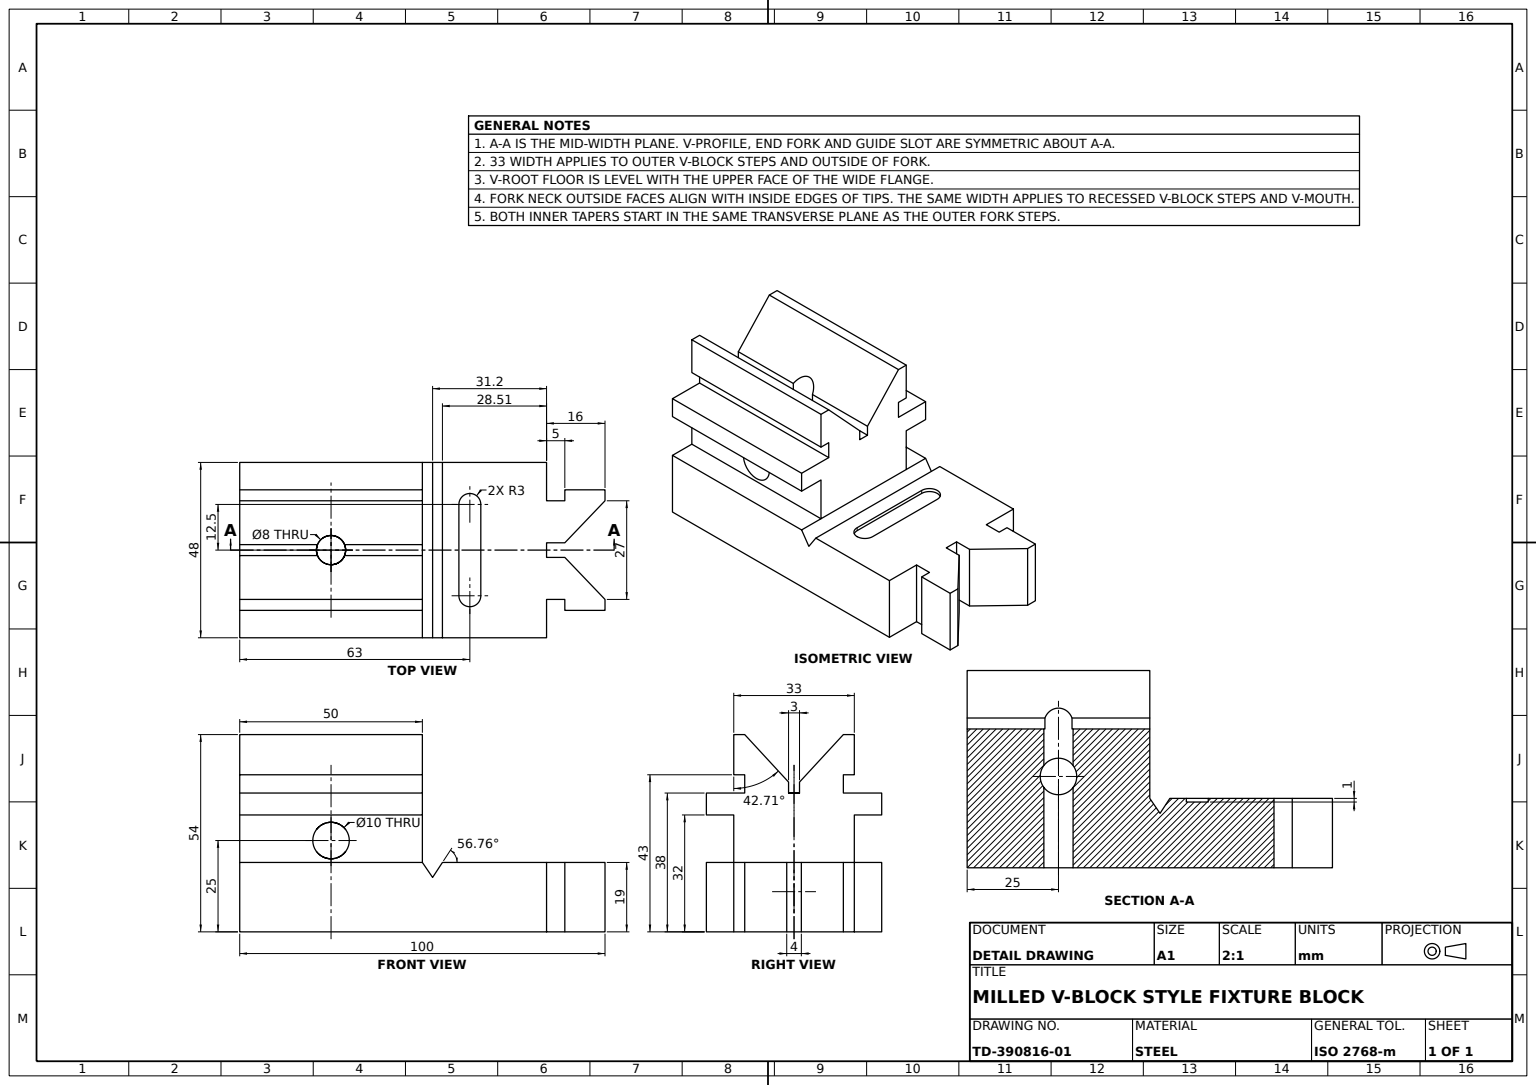
SolidWorks part; units mm, degrees
material "Plain Carbon Steel"
ref_plane "Front Plane" through (0, 0, 0) normal (0, 0, 1) x (1, 0, 0)
ref_plane "Top Plane" through (0, 0, 0) normal (0, 1, 0) x (1, 0, 0)
ref_plane "Right Plane" through (0, 0, 0) normal (1, 0, 0) x (0, 0, -1)
sketch "Base Block Profile" plane through (0, 0, 0) normal (0, 0, 1) x (1, 0, 0)
  line L0 (0, 0) -> (100, 0)
  line L1 (100, 0) -> (100, 19)
  line L2 (100, 19) -> (0, 19)
  line L8 (0, 0) -> (0, 19)
  dimension "D1" = 100
  dimension "D4" = 19
extrude "Base Block 100x19x48" add sketch "Base Block Profile" along normal mid plane 48
sketch "End Notch Profile" plane through (0, 19, 0) normal (0, 1, 0) x (1, 0, 0)
  line L0 (84, 24) -> (84, 13.5)
  line L1 (100, 24) -> (0, 24) construction
  line L2 (84, 13.5) -> (89, 13.5)
  line L3 (89, 13.5) -> (89, 16.5)
  line L4 (89, 16.5) -> (100, 16.5)
  line L5 (100, -24) -> (100, 24) construction
  line L7 (100, 13.5) -> (89, 2)
  line L8 (89, 2) -> (84, 2)
  line L9 (84, 2) -> (84, -2)
  line L10 (84, -2) -> (89, -2)
  line L11 (-4.806, 0) -> (110.2978, 0) construction
  line L12 (100, -13.5) -> (89, -2)
  line L13 (100, -16.5) -> (100, -13.5)
  line L14 (89, -16.5) -> (100, -16.5)
  line L15 (89, -13.5) -> (89, -16.5)
  line L16 (84, -13.5) -> (89, -13.5)
  line L17 (84, -24) -> (84, -13.5)
  line L18 (84, 24) -> (100, 24)
  line L19 (100, 24) -> (100, 16.5)
  line L20 (84, -24) -> (100, -24)
  line L21 (100, -24) -> (100, -16.5)
  line L22 (100, -13.5) -> (100, 13.5)
  line M17 (100, 24) -> (0, 24)
  line M19 (0, -24) -> (100, -24)
  line M20 (100, -24) -> (100, 24)
  dimension "D1" = 33
  dimension "D2" = 27
  dimension "D3" = 4
  dimension "D4" = 5
  dimension "D5" = 16
extrude "End Notches Cut" cut sketch "End Notch Profile" against normal mid plane 48 contours L17 L14 L15 L16 M19 M20 | L11 L9 L10 L12 M20 | L9 L11 L22 L7 L8 | L3 L4 L0 L2 M20 M17
sketch "Guide Slot Sketch" plane through (0, 19, 0) normal (0, 1, 0) x (1, 0, 0)
  line L0 (63, -12.5) -> (63, 12.5) construction
  line L1 (60, -12.5) -> (60, 12.5)
  line L2 (66, -12.5) -> (66, 12.5)
  arc A0 (60, -12.5) -> (66, -12.5) centre (63, -12.5) ccw
  arc A1 (66, 12.5) -> (60, 12.5) centre (63, 12.5) ccw
  point P2 (63, 0)
  dimension "D2" = 3
  dimension "D1" = 63
  dimension "D3" = 25
  dimension "D4" = 12.5
extrude "Guide Slot 63x3 Depth 1" cut sketch "Guide Slot Sketch" against normal blind 1
sketch "V-Block Body Profile" plane through (0, 0, 0) normal (-1, 0, 0) x (0, 0, 1)
  line L0 (-16.5, 19) -> (-16.5, 32)
  line L1 (24, 19) -> (-24, 19) construction
  line L2 (-16.5, 32) -> (-24, 32)
  line L3 (-24, 32) -> (-24, 38)
  line L4 (-24, 38) -> (-13.5, 38)
  line L5 (-13.5, 38) -> (-13.5, 43)
  line L6 (-13.5, 43) -> (-16.5, 43)
  line L7 (-16.5, 43) -> (-16.5, 54)
  line L8 (-16.5, 54) -> (-13.5, 54)
  line L9 (-13.5, 54) -> (-1.5, 41)
  line L10 (-1.5, 41) -> (-1.5, 38)
  line L11 (-1.5, 38) -> (1.5, 38)
  line L12 (0, -29.7) -> (0, 29.7) construction
  line L13 (1.5, 41) -> (1.5, 38)
  line L14 (13.5, 54) -> (1.5, 41)
  line L15 (16.5, 54) -> (13.5, 54)
  line L16 (16.5, 43) -> (16.5, 54)
  line L17 (13.5, 43) -> (16.5, 43)
  line L18 (13.5, 38) -> (13.5, 43)
  line L19 (24, 38) -> (13.5, 38)
  line L20 (24, 32) -> (24, 38)
  line L21 (16.5, 32) -> (24, 32)
  line L22 (16.5, 19) -> (16.5, 32)
  line L23 (-16.5, 19) -> (16.5, 19)
  line L24 (24, 0) -> (-24, 0) construction
  point P17 (0, 38)
  point P30 (16.5, 25.5)
  dimension "D1" = 48
  dimension "D2" = 27
  dimension "D3" = 33
  dimension "D4" = 43
  dimension "D5" = 54
  dimension "D6" = 3
  dimension "D7" = 38
  dimension "D8" = 32
  dimension "D9" = 33
  dimension "D10" = 3
  dimension "D11" = 38
extrude "V-Block Body" add sketch "V-Block Body Profile" against normal blind 50
sketch "V-Groove Sketch" plane through (0, 0, 24) normal (0, 0, 1) x (1, 0, 0)
  line L0 (50, 19) -> (52.8019, 14.8956)
  line L1 (52.8019, 14.8956) -> (55.4918, 19)
  line L2 (84, 19) -> (0, 19) construction
  line L3 (55.4918, 19) -> (50, 19)
  line L4 (84, 0) -> (84, 19) construction
  line L5 (0, 0) -> (84, 0) construction
  dimension "D1" = 28.5082
  dimension "D2" = 31.1981
  dimension "D3" = 14.8956
extrude "V-Groove Cut" cut sketch "V-Groove Sketch" against normal blind 60
sketch "Cross Hole Ø8 Sketch" plane through (0, 38, 0) normal (0, 1, 0) x (1, 0, 0)
  line L0 (0, -13.5) -> (0, -1.5) construction
  line L1 (50, 24) -> (0, 24) construction
  circle A0 centre (25, 0) radius 4
  dimension "D1" = 8
  dimension "D2" = 25
  dimension "D3" = 24
extrude "Cross Hole Ø8" cut sketch "Cross Hole Ø8 Sketch" against normal mid plane 110
sketch "Hole Ø10 Sketch" plane through (0, 0, 24) normal (0, 0, 1) x (1, 0, 0)
  line L0 (0, 0) -> (84, 0) construction
  line L1 (0, 19) -> (0, 32) construction
  circle A0 centre (25, 25) radius 5
  dimension "D1" = 10
  dimension "D2" = 25
  dimension "D3" = 25
extrude "Hole Ø10" cut sketch "Hole Ø10 Sketch" against normal blind 60
